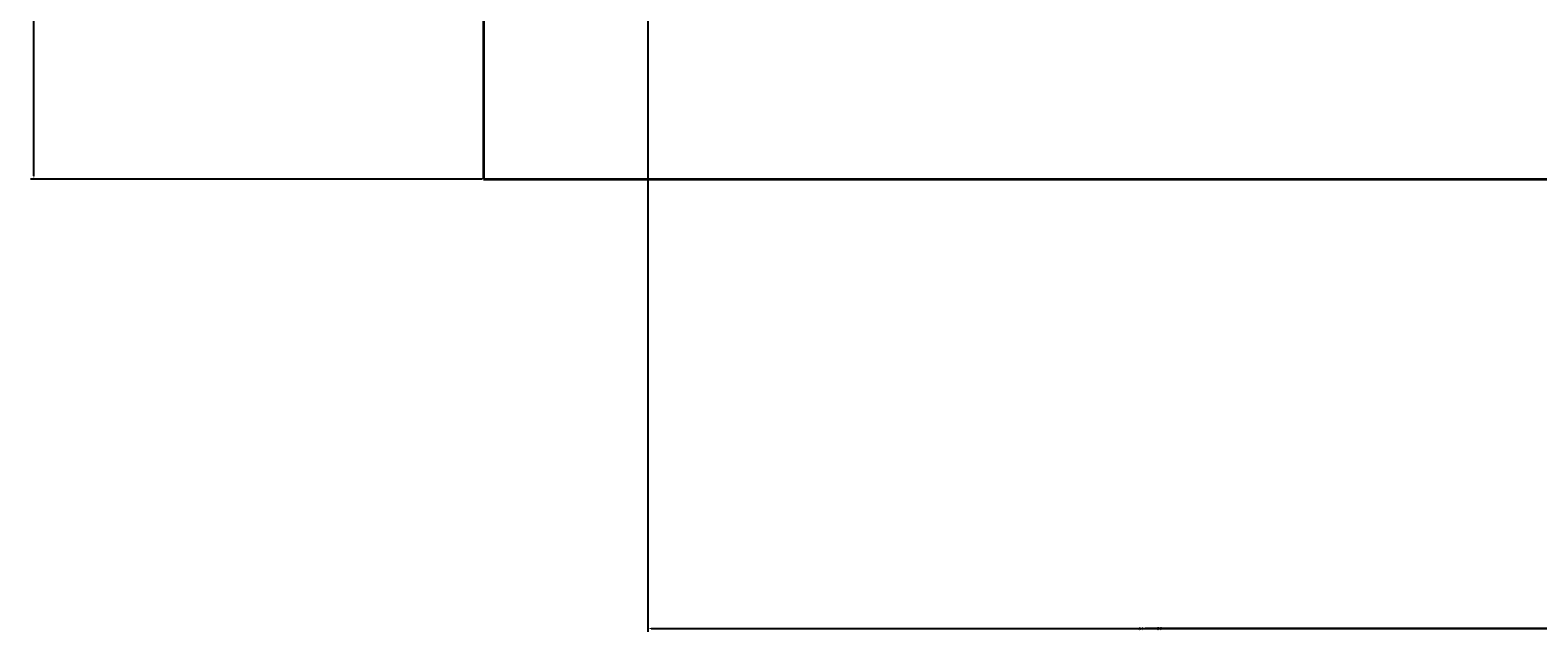
# Model space of a CAD drawing. Units: inches. Extents: x 8049 to 8459, y 820 to 1350.
# Tile 1 of 25: x 8050 to 8132, y 820 to 853. Entities that reach past the tile are written whole.
import ezdxf

# ---------------------------------------------------------------- set-up
doc = ezdxf.new("R2010")
doc.units = ezdxf.units.IN
doc.header["$MEASUREMENT"] = 0
doc.layers.add('A-ANNO-DIMS', color=2, linetype='Continuous', lineweight=18)
doc.layers.add('C-SITE-WALL', color=7, linetype='Continuous', lineweight=35)
doc.styles.get("Standard").update_dxf_attribs({"font": 'arial.ttf'})
doc.dimstyles.get("Standard").update_dxf_attribs({"dimtxt": 0.18, "dimasz": 0.18, "dimexe": 0.18, "dimexo": 0.0625, "dimgap": 0.09, "dimtad": 0, "dimtih": 1, "dimtoh": 1, "dimdec": 4, "dimzin": 0, "dimdsep": 46, "dimtxsty": 'Standard', "dimcen": 0.09, "dimadec": 0, "dimazin": 0, "dimtfac": 1, "dimtdec": 4, "dimtofl": 0, "dimtmove": 0, "dimatfit": 3, "dimfxl": 1, "dimtolj": 1, "dimtzin": 0, "dimarcsym": 0})

# ---------------------------------------------------------------- blocks, each defined once
blk = doc.blocks.new('*D50')
at = {"layer": 'A-ANNO-DIMS', "color": 0, "lineweight": -2, "transparency": 16777216}
for p, q in [((8083.335, 1045.871), (8049.617, 1045.871)), ((8049.797, 1045.691), (8049.797, 945.553)), ((8049.797, 845.051), (8049.797, 945.189)), ((8074.335, 844.871), (8049.617, 844.871))]:
    blk.add_line(p, q, dxfattribs=at)
at = {"layer": 'A-ANNO-DIMS', "color": 0, "transparency": 16777216}
for points in [[(8049.767, 1045.691), (8049.827, 1045.691), (8049.797, 1045.871)], [(8049.767, 845.051), (8049.827, 845.051), (8049.797, 844.871)]]:
    blk.add_solid(points, dxfattribs=at)
at = {"layer": 'Defpoints', "color": 0, "transparency": 16777216}
for p in [(8049.797, 1045.871), (8083.397, 1045.871), (8074.397, 844.871)]:
    blk.add_point(p, dxfattribs=at)
at = {"layer": 'A-ANNO-DIMS', "color": 0, "transparency": 16777216, "insert": (8049.797, 945.371), "char_height": 0.18, "attachment_point": 5}
blk.add_mtext('\\A1;201', dxfattribs=at)
blk = doc.blocks.new('*D70')
at = {"layer": 'A-ANNO-DIMS', "color": 0, "lineweight": -2, "transparency": 16777216}
for p, q in [((8083.397, 1045.808), (8083.397, 820.091)), ((8137.397, 1045.808), (8137.397, 820.091)), ((8083.577, 820.271), (8110.179, 820.271)), ((8137.217, 820.271), (8110.616, 820.271))]:
    blk.add_line(p, q, dxfattribs=at)
at = {"layer": 'A-ANNO-DIMS', "color": 0, "transparency": 16777216}
for points in [[(8083.577, 820.301), (8083.577, 820.241), (8083.397, 820.271)], [(8137.217, 820.301), (8137.217, 820.241), (8137.397, 820.271)]]:
    blk.add_solid(points, dxfattribs=at)
at = {"layer": 'Defpoints', "color": 0, "transparency": 16777216}
for p in [(8083.397, 1045.871), (8137.397, 1045.871), (8083.397, 820.271)]:
    blk.add_point(p, dxfattribs=at)
at = {"layer": 'A-ANNO-DIMS', "color": 0, "transparency": 16777216, "insert": (8110.397, 820.271), "char_height": 0.18, "attachment_point": 5}
blk.add_mtext('\\A1;54', dxfattribs=at)
blk = doc.blocks.new('*D76')
at = {"layer": 'A-ANNO-DIMS', "color": 0, "lineweight": -2, "transparency": 16777216}
for p, q in [((8083.397, 1054.808), (8083.397, 820.091)), ((8299.397, 1054.808), (8299.397, 820.091)), ((8083.577, 820.271), (8191.107, 820.271)), ((8299.217, 820.271), (8191.688, 820.271))]:
    blk.add_line(p, q, dxfattribs=at)
at = {"layer": 'A-ANNO-DIMS', "color": 0, "transparency": 16777216}
for points in [[(8083.577, 820.301), (8083.577, 820.241), (8083.397, 820.271)], [(8299.217, 820.301), (8299.217, 820.241), (8299.397, 820.271)]]:
    blk.add_solid(points, dxfattribs=at)
at = {"layer": 'Defpoints', "color": 0, "transparency": 16777216}
for p in [(8083.397, 1054.871), (8299.397, 1054.871), (8299.397, 820.271)]:
    blk.add_point(p, dxfattribs=at)
at = {"layer": 'A-ANNO-DIMS', "color": 0, "transparency": 16777216, "insert": (8191.397, 820.271), "char_height": 0.18, "attachment_point": 5}
blk.add_mtext('\\A1;216', dxfattribs=at)
blk = doc.blocks.new('*D88')
at = {"layer": 'A-ANNO-DIMS', "color": 0, "lineweight": -2, "transparency": 16777216}
for p, q in [((8083.397, 1162.808), (8083.397, 820.091)), ((8139.397, 1162.808), (8139.397, 820.091)), ((8083.577, 820.271), (8111.179, 820.271)), ((8139.217, 820.271), (8111.616, 820.271))]:
    blk.add_line(p, q, dxfattribs=at)
at = {"layer": 'A-ANNO-DIMS', "color": 0, "transparency": 16777216}
for points in [[(8083.577, 820.301), (8083.577, 820.241), (8083.397, 820.271)], [(8139.217, 820.301), (8139.217, 820.241), (8139.397, 820.271)]]:
    blk.add_solid(points, dxfattribs=at)
at = {"layer": 'Defpoints', "color": 0, "transparency": 16777216}
for p in [(8083.397, 1162.871), (8139.397, 1162.871), (8139.397, 820.271)]:
    blk.add_point(p, dxfattribs=at)
at = {"layer": 'A-ANNO-DIMS', "color": 0, "transparency": 16777216, "insert": (8111.397, 820.271), "char_height": 0.18, "attachment_point": 5}
blk.add_mtext('\\A1;56', dxfattribs=at)

msp = doc.modelspace()

# ---------------------------------------------------------------- linework, layer by layer
at = {"layer": 'C-SITE-WALL'}
for p, q in [((8074.3974, 1324.8706), (8074.3974, 844.8706)), ((8074.3974, 844.8706), (8219.8974, 844.8706))]:
    msp.add_line(p, q, dxfattribs=at)

# ---------------------------------------------------------------- dimensions: what is measured, and where the dimension line sits
at = {"layer": 'A-ANNO-DIMS'}
for base, p1, p2, picture, middle in [((8139.3974, 820.2706), (8083.3974, 1162.8706), (8139.3974, 1162.8706), '*D88', (8111.3974, 820.2706)), ((8299.3974, 820.2706), (8083.3974, 1054.8706), (8299.3974, 1054.8706), '*D76', (8191.3974, 820.2706)), ((8083.3974, 820.2706), (8137.3974, 1045.8706), (8083.3974, 1045.8706), '*D70', (8110.3974, 820.2706))]:
    dim = msp.add_linear_dim(base=base, p1=p1, p2=p2, dimstyle='Standard', override={"dimdec": 0, "dimlfac": 1, "dimrnd": 0, "dimzin": 0, "dimdsep": 46, "dimlunit": 2}, dxfattribs=at)
    dim.commit()
    dim.dimension.update_dxf_attribs({"geometry": picture, "text_midpoint": middle})
dim = msp.add_linear_dim(base=(8049.7974, 1045.8706), p1=(8074.3974, 844.8706), p2=(8083.3974, 1045.8706), angle=90, dimstyle='Standard', override={"dimdec": 0, "dimlfac": 1, "dimrnd": 0, "dimzin": 0, "dimdsep": 46, "dimlunit": 2}, dxfattribs=at)
dim.commit()
dim.dimension.update_dxf_attribs({"geometry": '*D50', "text_midpoint": (8049.7974, 945.3706)})

doc.saveas('drawing.dxf')
